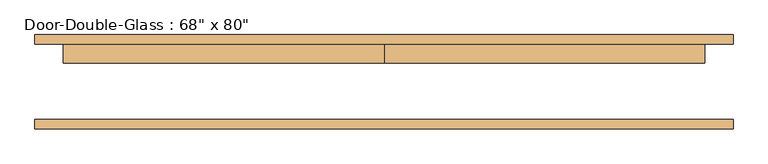
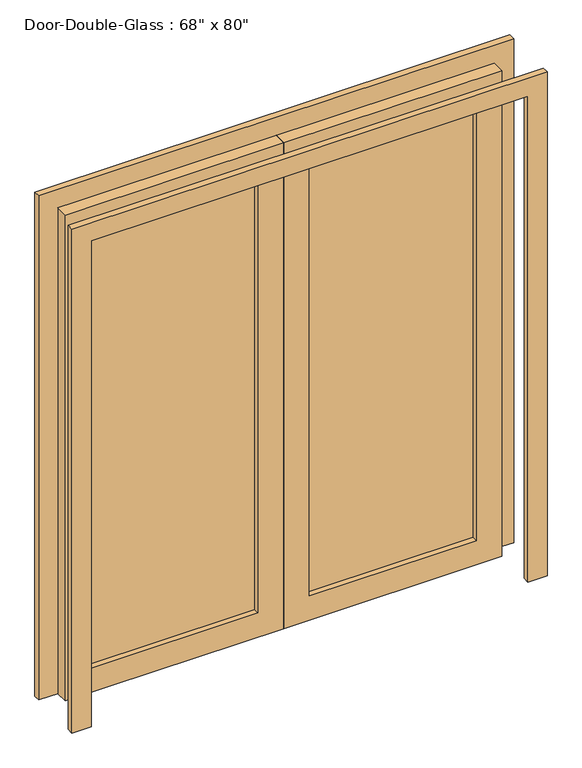
"""IFC4 building model written with IfcOpenShell, lengths in millimetres: door geometry."""

from ifc_helpers import new_model, si_unit, frame, origin, place, context, project, spatial, polyline, outline, extrude, source, transform, mapped, element, save


def door_10418eaf(model_context):
    return source(origin(), model_context, "Body", "SweptSolid", [
        extrude(outline(polyline([(2032.0, -863.6), (0.0, -863.6), (0.0, 0.0), (2032.0, 0.0), (2032.0, -863.6)]), holes=[polyline([(1930.4, -762.0), (1930.4, -101.6), (101.6, -101.6), (101.6, -762.0), (1930.4, -762.0)])]), frame((0.0, 53.18125, 0.0), z_axis=(0.0, 1.0, 0.0), x_axis=(0.0, 0.0, 1.0)), (0.0, 0.0, 1.0), 50.8),
        extrude(outline(polyline([(2032.0, 863.6), (2032.0, 0.0), (0.0, 0.0), (0.0, 863.6), (2032.0, 863.6)]), holes=[polyline([(1930.4, 762.0), (101.6, 762.0), (101.6, 101.6), (1930.4, 101.6), (1930.4, 762.0)])]), frame((0.0, 53.18125, 0.0), z_axis=(0.0, 1.0, 0.0), x_axis=(0.0, 0.0, 1.0)), (0.0, 0.0, 1.0), 50.8),
        extrude(outline(polyline([(101.6, 81.75625), (762.0, 81.75625), (762.0, 75.40625), (101.6, 75.40625), (101.6, 81.75625)])), frame((0.0, 0.0, 101.6), z_axis=(0.0, 0.0, 1.0), x_axis=(1.0, 0.0, 0.0)), (0.0, 0.0, 1.0), 1828.8),
        extrude(outline(polyline([(-762.0, 81.75625), (-101.6, 81.75625), (-101.6, 75.40625), (-762.0, 75.40625), (-762.0, 81.75625)])), frame((0.0, 0.0, 101.6), z_axis=(0.0, 0.0, 1.0), x_axis=(1.0, 0.0, 0.0)), (0.0, 0.0, 1.0), 1828.8),
        extrude(outline(polyline([(0.0, 939.8), (2108.2, 939.8), (2108.2, -939.8), (0.0, -939.8), (0.0, -863.6), (2032.0, -863.6), (2032.0, 863.6), (0.0, 863.6), (0.0, 939.8)])), frame((0.0, 103.98125, 0.0), z_axis=(0.0, 1.0, 0.0), x_axis=(0.0, 0.0, 1.0)), (0.0, 0.0, 1.0), 25.4),
        extrude(outline(polyline([(0.0, 939.8), (2108.2, 939.8), (2108.2, -939.8), (0.0, -939.8), (0.0, -863.6), (2032.0, -863.6), (2032.0, 863.6), (0.0, 863.6), (0.0, 939.8)])), frame((0.0, -124.61875, 0.0), z_axis=(0.0, 1.0, 0.0), x_axis=(0.0, 0.0, 1.0)), (0.0, 0.0, 1.0), 25.4),
    ])


if __name__ == "__main__":
    model = new_model("IFC4")
    model_context = context("Model", 3, world=origin())
    ifc_project = project(units=[si_unit("LENGTHUNIT", "METRE", prefix="MILLI")], contexts=[model_context])
    site = spatial("IfcSite", under=ifc_project)
    building = spatial("IfcBuilding", under=site)
    placement = place(None, origin())
    door_shape = door_10418eaf(model_context)
    element("IfcDoor", 1, ObjectType="Door-Double-Glass : 68\" x 80\"", at=placement, inside=building, context=model_context, shape_type="MappedRepresentation", body=[
        mapped(door_shape, transform((0.0, 0.0, 0.0), x_axis=(1.0, 0.0, 0.0), y_axis=(0.0, 1.0, 0.0), z_axis=(0.0, 0.0, 1.0))),
    ])
    save(model, "model.ifc")

# Revit data of these elements
# Type "Door-Double-Glass : 68\" x 80\""
#   Type Mark = "8"
#   Construction Type Id = "opn-d45"
#   Assembly Code = "C1020"
#   Analytic Construction = "Wood frame, double glass door "
#   W = 2' - 10"
#   Thickness = 0' - 2"
#   Thermal Resistance (R) = 1.8150 (h·ft²·°F)/BTU
#   Swing Angle [instance default] = 90.00°
#   Heat Transfer Coefficient (U) = 0.5510 BTU/(h·ft²·°F)
#   Height = 6' - 8"
#   Bottom Rail = 0' - 4"
#   Top Rail = 0' - 4"
#   Stiles = 0' - 4"
#   Trim Projection = 0' - 1"
#   Trim Width = 0' - 3"
#   Width = 5' - 8"
#   Define Thermal Properties by = 1
#   Glazing = Glass
#   Panel Material = Wood - Birch - Solid Stained Light Low Gloss
#   Trim Material = Paint - Sienna
#   Visual Light Transmittance = 0
#   Solar Heat Gain Coefficient = 0
#   Function = (empty or 0)
#   Wall Closure = (empty or 0)
# Element 1 (IfcDoor, "Door-Double-Glass : 68\" x 80\"")
#   Materials on its faces: "Wood - Birch - Solid Stained Light Low Gloss", "Paint - Sienna", "Glass"
# Materials
#   "Glass": class "Glass", colour RGB 0 128 192, transparency 0.75, Description = "Soda Lime Glass", Cost = 0
#   "Wood - Birch - Solid Stained Light Low Gloss": class "Wood", colour RGB 210 159 95, transparency 0, Cost = 0
#   "Paint - Sienna": colour RGB 118 70 51, transparency 0, Cost = 0
